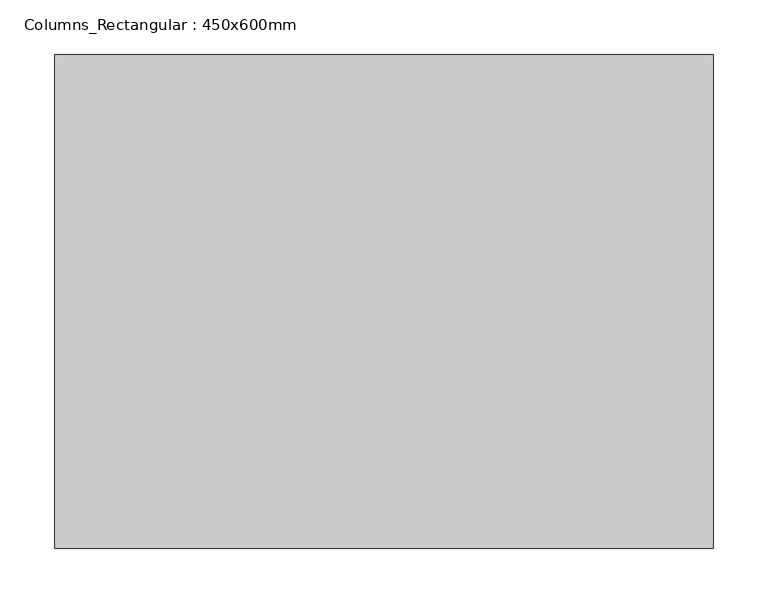
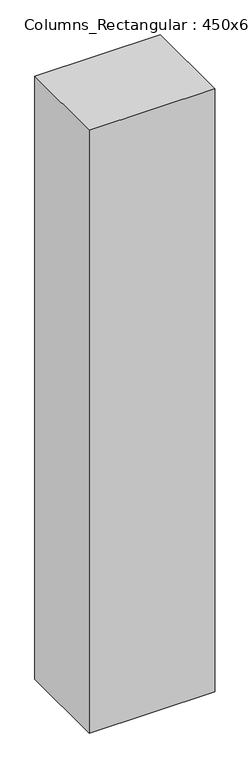
"""IFC4 building model written with IfcOpenShell, lengths in millimetres: column geometry, Columns_Rectangular : 450x600mm."""

from ifc_helpers import new_model, si_unit, frame, origin, place, context, project, spatial, polyline, outline, extrude, source, transform, mapped, element, save


def columns_rectangular_450x600mm_2bb2af66(model_context):
    return source(origin(), model_context, "Body", "SweptSolid", [
        extrude(outline(polyline([(300.0, 225.0), (300.0, -225.0), (-300.0, -225.0), (-300.0, 225.0), (300.0, 225.0)])), frame((0.0, 0.0, 487.68), z_axis=(0.0, 0.0, 1.0), x_axis=(1.0, 0.0, 0.0)), (0.0, 0.0, 1.0), 3048.0),
    ])


if __name__ == "__main__":
    model = new_model("IFC4")
    model_context = context("Model", 3, world=origin())
    ifc_project = project(units=[si_unit("LENGTHUNIT", "METRE", prefix="MILLI")], contexts=[model_context])
    site = spatial("IfcSite", under=ifc_project)
    building = spatial("IfcBuilding", under=site)
    placement = place(None, origin())
    columns_rectangular_450x600mm_shape = columns_rectangular_450x600mm_2bb2af66(model_context)
    element("IfcColumn", 1, ObjectType="Columns_Rectangular : 450x600mm", at=placement, inside=building, context=model_context, shape_type="MappedRepresentation", body=[
        mapped(columns_rectangular_450x600mm_shape, transform((0.0, 0.0, 0.0), x_axis=(1.0, 0.0, 0.0), y_axis=(0.0, 1.0, 0.0), z_axis=(0.0, 0.0, 1.0))),
    ])
    save(model, "model.ifc")

# Revit data of these elements
# Type "Columns_Rectangular : 450x600mm"
#   Keynote = "G"
#   Depth = 1.476378 ft
#   Offset Base = 0.0 ft
#   Offset Top = 0.0 ft
#   Width = 1.968504 ft
#   Material = none
